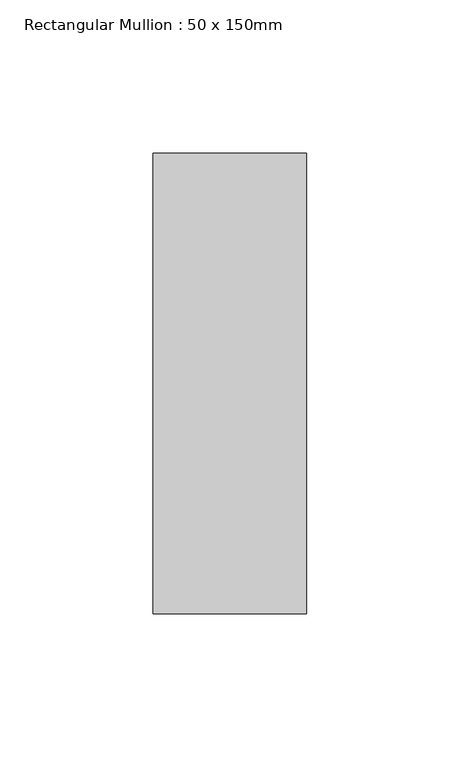
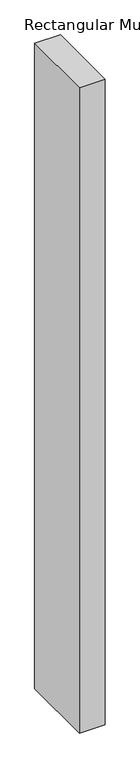
"""IFC4 building model written with IfcOpenShell, lengths in millimetres: member geometry, Rectangular Mullion : 50 x 150mm."""

from ifc_helpers import new_model, si_unit, frame, origin, place, context, project, spatial, polyline, outline, extrude, source, transform, mapped, element, save


def rectangular_mullion_50_x_150mm_e4d4a7e6(model_context):
    return source(origin(), model_context, "Body", "SweptSolid", [
        extrude(outline(polyline([(0.0, 75.0), (0.0, -75.0), (-50.0, -75.0), (-50.0, 75.0), (0.0, 75.0)])), frame((0.0, 0.0, -1321.6), z_axis=(0.0, 0.0, 1.0), x_axis=(1.0, 0.0, 0.0)), (0.0, 0.0, 1.0), 1321.6),
    ])


if __name__ == "__main__":
    model = new_model("IFC4")
    model_context = context("Model", 3, world=origin())
    ifc_project = project(units=[si_unit("LENGTHUNIT", "METRE", prefix="MILLI")], contexts=[model_context])
    site = spatial("IfcSite", under=ifc_project)
    building = spatial("IfcBuilding", under=site)
    placement = place(None, origin())
    rectangular_mullion_50_x_150mm_shape = rectangular_mullion_50_x_150mm_e4d4a7e6(model_context)
    element("IfcMember", 1, ObjectType="Rectangular Mullion : 50 x 150mm", at=placement, inside=building, context=model_context, shape_type="MappedRepresentation", body=[
        mapped(rectangular_mullion_50_x_150mm_shape, transform((0.0, 0.0, 0.0), x_axis=(1.0, 0.0, 0.0), y_axis=(0.0, 1.0, 0.0), z_axis=(0.0, 0.0, 1.0))),
    ])
    save(model, "model.ifc")

# Revit data of these elements
# Type "Rectangular Mullion : 50 x 150mm"
#   built-in parameter 1007304 = 0.492126 (stored number, unit not read)
#   built-in parameter 1007301 = 0.082021 (stored number, unit not read)
#   built-in parameter 1007300 = 0.082021 (stored number, unit not read)
# Element 1 (IfcMember, "Rectangular Mullion : 50 x 150mm")
#   Materials on its faces: "Aluminium"
# Materials
#   "Aluminium": class "Metal", colour RGB 247 247 247, transparency 0, Description = "Aluminium 6061", Cost = 0
